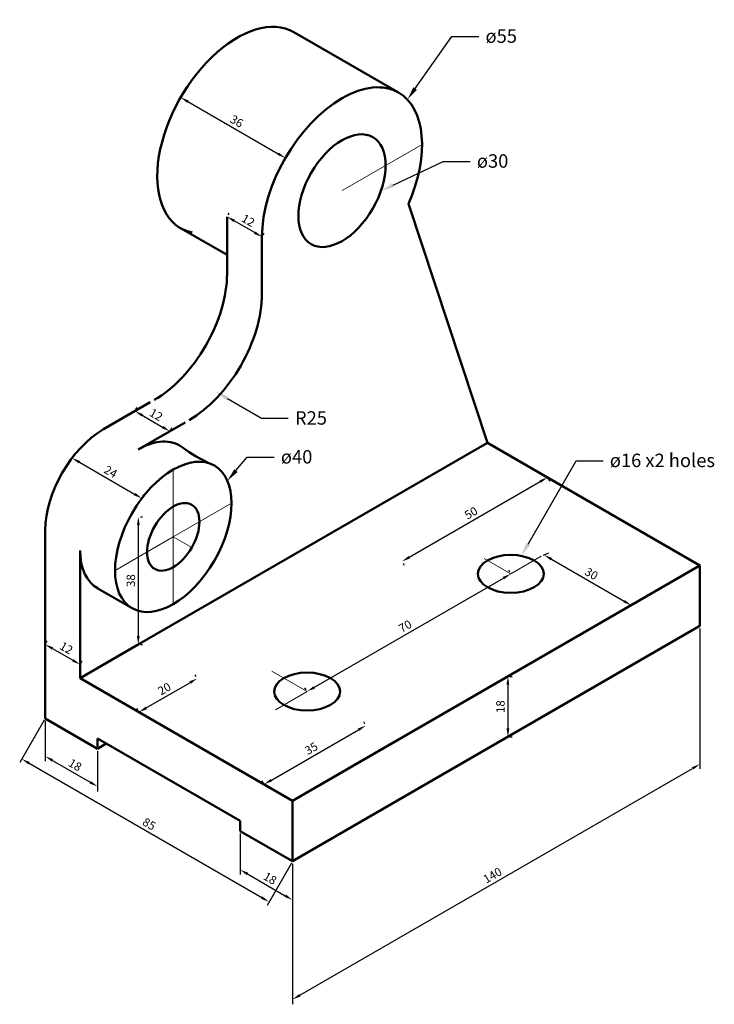
# Model space of a CAD drawing. Units: millimetres. Extents: x 2139 to 2346, y 2028 to 2321.
import ezdxf
from ezdxf import colors
from ezdxf.entities.mleader import LeaderData, LeaderLine
from ezdxf.math import Vec2, Vec3

# ---------------------------------------------------------------- set-up
doc = ezdxf.new("R2010")
doc.units = ezdxf.units.MM
doc.linetypes.add('CENTER', pattern=[50.8, 31.75, -6.35, 6.35, -6.35])
for name, color, linetype, lineweight in [('M-CNTR', 1, 'CENTER', 18), ('M-DIMS', 2, 'Continuous', 25), ('M-OUTL', 7, 'Continuous', 50), ('M-TEXT', 3, 'Continuous', 25)]:
    doc.layers.add(name, color=color, linetype=linetype, lineweight=lineweight)
doc.styles.get("Standard").update_dxf_attribs({"font": 'arial.ttf'})
doc.dimstyles.new('ISO-25', dxfattribs={"dimtxt": 2.5, "dimasz": 2.5, "dimexe": 1.25, "dimexo": 0.625, "dimtad": 1, "dimtxsty": 'Standard', "dimcen": 2.5, "dimadec": 0, "dimazin": 0, "dimtfac": 1, "dimtmove": 0, "dimatfit": 3, "dimfxl": 1, "dimarcsym": 0})

# ---------------------------------------------------------------- blocks, each defined once
blk = doc.blocks.new('*D1')
at = {"layer": 'Defpoints', "color": 0, "transparency": 16777216}
for p in [(2186.84, 2297.97), (2218.02, 2279.97), (2218.02, 2279.97)]:
    blk.add_point(p, dxfattribs=at)
at = {"layer": 'M-DIMS', "color": 0, "lineweight": -2, "transparency": 16777216}
for p, q in [((2187.16, 2298.51), (2187.47, 2299.05)), ((2189.01, 2296.72), (2215.86, 2281.22)), ((2218.33, 2280.51), (2218.65, 2281.05))]:
    blk.add_line(p, q, dxfattribs=at)
at = {"layer": 'M-DIMS', "color": 0, "transparency": 16777216}
for points in [[(2189.22, 2297.08), (2188.8, 2296.36), (2186.84, 2297.97)], [(2216.06, 2281.58), (2215.65, 2280.86), (2218.02, 2279.97)]]:
    blk.add_solid(points, dxfattribs=at)
at = {"layer": 'M-DIMS', "color": 0, "transparency": 16777216, "insert": (2203.38, 2290.62), "char_height": 2.5, "attachment_point": 5, "rotation": 330}
blk.add_mtext('36', dxfattribs=at)
blk = doc.blocks.new('*D2')
at = {"layer": 'Defpoints', "color": 0, "transparency": 16777216}
for p in [(2296.01, 2184.94), (2296.01, 2184.94), (2252.71, 2159.94)]:
    blk.add_point(p, dxfattribs=at)
at = {"layer": 'M-DIMS', "color": 0, "lineweight": -2, "transparency": 16777216}
for p, q in [((2254.87, 2161.19), (2293.84, 2183.69)), ((2296.32, 2184.4), (2296.63, 2183.86)), ((2253.02, 2159.4), (2253.33, 2158.86))]:
    blk.add_line(p, q, dxfattribs=at)
at = {"layer": 'M-DIMS', "color": 0, "transparency": 16777216}
for points in [[(2293.64, 2184.05), (2294.05, 2183.33), (2296.01, 2184.94)], [(2254.66, 2161.55), (2255.08, 2160.83), (2252.71, 2159.94)]]:
    blk.add_solid(points, dxfattribs=at)
at = {"layer": 'M-DIMS', "color": 0, "transparency": 16777216, "insert": (2273.41, 2174.09), "char_height": 2.5, "attachment_point": 5, "rotation": 30}
blk.add_mtext('50', dxfattribs=at)
blk = doc.blocks.new('*D3')
at = {"layer": 'Defpoints', "color": 0, "transparency": 16777216}
for p in [(2241.97, 2111.14), (2241.97, 2111.14), (2211.66, 2093.64)]:
    blk.add_point(p, dxfattribs=at)
at = {"layer": 'M-DIMS', "color": 0, "lineweight": -2, "transparency": 16777216}
for p, q in [((2241.66, 2111.68), (2241.35, 2112.22)), ((2213.83, 2094.89), (2239.81, 2109.89)), ((2211.35, 2094.18), (2211.04, 2094.72))]:
    blk.add_line(p, q, dxfattribs=at)
at = {"layer": 'M-DIMS', "color": 0, "transparency": 16777216}
for points in [[(2239.6, 2110.25), (2240.01, 2109.53), (2241.97, 2111.14)], [(2213.62, 2095.25), (2214.03, 2094.53), (2211.66, 2093.64)]]:
    blk.add_solid(points, dxfattribs=at)
at = {"layer": 'M-DIMS', "color": 0, "transparency": 16777216, "insert": (2225.86, 2104.04), "char_height": 2.5, "attachment_point": 5, "rotation": 30}
blk.add_mtext('35', dxfattribs=at)
blk = doc.blocks.new('*D4')
at = {"layer": 'Defpoints', "color": 0, "transparency": 16777216}
for p in [(2146.53, 2113.25), (2162.12, 2104.25), (2162.12, 2092.99)]:
    blk.add_point(p, dxfattribs=at)
at = {"layer": 'M-DIMS', "color": 0, "lineweight": -2, "transparency": 16777216}
for p, q in [((2146.53, 2112.52), (2146.53, 2100.54)), ((2162.12, 2103.52), (2162.12, 2091.54)), ((2148.69, 2100.74), (2159.95, 2094.24))]:
    blk.add_line(p, q, dxfattribs=at)
at = {"layer": 'M-DIMS', "color": 0, "transparency": 16777216}
for points in [[(2148.9, 2101.1), (2148.48, 2100.37), (2146.53, 2101.99)], [(2160.16, 2094.6), (2159.74, 2093.87), (2162.12, 2092.99)]]:
    blk.add_solid(points, dxfattribs=at)
at = {"layer": 'M-DIMS', "color": 0, "transparency": 16777216, "insert": (2155.27, 2099.13), "char_height": 2.5, "attachment_point": 5, "rotation": 330}
blk.add_mtext('18', dxfattribs=at)
blk = doc.blocks.new('*D5')
at = {"layer": 'Defpoints', "color": 0, "transparency": 16777216}
for p in [(2204.55, 2079.75), (2220.14, 2070.75), (2220.14, 2059.24)]:
    blk.add_point(p, dxfattribs=at)
at = {"layer": 'M-DIMS', "color": 0, "lineweight": -2, "transparency": 16777216}
for p, q in [((2204.55, 2079.02), (2204.55, 2066.8)), ((2220.14, 2070.02), (2220.14, 2057.8)), ((2206.72, 2066.99), (2217.97, 2060.49))]:
    blk.add_line(p, q, dxfattribs=at)
at = {"layer": 'M-DIMS', "color": 0, "transparency": 16777216}
for points in [[(2206.92, 2067.35), (2206.51, 2066.63), (2204.55, 2068.24)], [(2218.18, 2060.85), (2217.77, 2060.13), (2220.14, 2059.24)]]:
    blk.add_solid(points, dxfattribs=at)
at = {"layer": 'M-DIMS', "color": 0, "transparency": 16777216, "insert": (2213.3, 2065.39), "char_height": 2.5, "attachment_point": 5, "rotation": 330}
blk.add_mtext('18', dxfattribs=at)
blk = doc.blocks.new('*D6')
at = {"layer": 'Defpoints', "color": 0, "transparency": 16777216}
for p in [(2341.38, 2140.75), (2341.38, 2099.64), (2220.14, 2070.75)]:
    blk.add_point(p, dxfattribs=at)
at = {"layer": 'M-DIMS', "color": 0, "lineweight": -2, "transparency": 16777216}
for p, q in [((2341.38, 2140.02), (2341.38, 2098.2)), ((2222.3, 2030.89), (2339.22, 2098.39)), ((2220.14, 2070.02), (2220.14, 2028.2))]:
    blk.add_line(p, q, dxfattribs=at)
at = {"layer": 'M-DIMS', "color": 0, "transparency": 16777216}
for points in [[(2339.01, 2098.75), (2339.43, 2098.03), (2341.38, 2099.64)], [(2222.1, 2031.25), (2222.51, 2030.53), (2220.14, 2029.64)]]:
    blk.add_solid(points, dxfattribs=at)
at = {"layer": 'M-DIMS', "color": 0, "transparency": 16777216, "insert": (2279.81, 2066.29), "char_height": 2.5, "attachment_point": 5, "rotation": 30}
blk.add_mtext('140', dxfattribs=at)
blk = doc.blocks.new('*D7')
at = {"layer": 'Defpoints', "color": 0, "transparency": 16777216}
for p in [(2294.14, 2161.47), (2320.12, 2146.47), (2320.98, 2146.87)]:
    blk.add_point(p, dxfattribs=at)
at = {"layer": 'M-DIMS', "color": 0, "lineweight": -2, "transparency": 16777216}
for p, q in [((2294.83, 2161.79), (2296.39, 2162.52)), ((2297.17, 2160.62), (2318.82, 2148.12)), ((2320.81, 2146.79), (2322.37, 2147.52))]:
    blk.add_line(p, q, dxfattribs=at)
at = {"layer": 'M-DIMS', "color": 0, "transparency": 16777216}
for points in [[(2297.38, 2160.98), (2296.96, 2160.26), (2295, 2161.87)], [(2319.03, 2148.48), (2318.61, 2147.76), (2320.98, 2146.87)]]:
    blk.add_solid(points, dxfattribs=at)
at = {"layer": 'M-DIMS', "color": 0, "transparency": 16777216, "insert": (2308.94, 2156.02), "char_height": 2.5, "attachment_point": 5, "rotation": 330}
blk.add_mtext('30', dxfattribs=at)
blk = doc.blocks.new('*D8')
at = {"layer": 'Defpoints', "color": 0, "transparency": 16777216}
for p in [(2173.24, 2204.67), (2183.63, 2198.67), (2183.63, 2198.67)]:
    blk.add_point(p, dxfattribs=at)
at = {"layer": 'M-DIMS', "color": 0, "lineweight": -2, "transparency": 16777216}
for p, q in [((2173.55, 2205.21), (2173.87, 2205.75)), ((2175.41, 2203.42), (2181.47, 2199.92)), ((2183.95, 2199.21), (2184.26, 2199.75))]:
    blk.add_line(p, q, dxfattribs=at)
at = {"layer": 'M-DIMS', "color": 0, "transparency": 16777216}
for points in [[(2175.62, 2203.78), (2175.2, 2203.06), (2173.24, 2204.67)], [(2181.68, 2200.28), (2181.26, 2199.56), (2183.63, 2198.67)]]:
    blk.add_solid(points, dxfattribs=at)
at = {"layer": 'M-DIMS', "color": 0, "transparency": 16777216, "insert": (2179.38, 2203.3), "char_height": 2.5, "attachment_point": 5, "rotation": 330}
blk.add_mtext('12', dxfattribs=at)
blk = doc.blocks.new('*D9')
at = {"layer": 'Defpoints', "color": 0, "transparency": 16777216}
for p in [(2154.52, 2190.72), (2175.31, 2178.72), (2175.31, 2178.72)]:
    blk.add_point(p, dxfattribs=at)
at = {"layer": 'M-DIMS', "color": 0, "lineweight": -2, "transparency": 16777216}
for p, q in [((2154.83, 2191.26), (2155.15, 2191.8)), ((2156.69, 2189.47), (2173.14, 2179.97)), ((2175.62, 2179.26), (2175.93, 2179.8))]:
    blk.add_line(p, q, dxfattribs=at)
at = {"layer": 'M-DIMS', "color": 0, "transparency": 16777216}
for points in [[(2156.9, 2189.83), (2156.48, 2189.1), (2154.52, 2190.72)], [(2173.35, 2180.33), (2172.93, 2179.6), (2175.31, 2178.72)]]:
    blk.add_solid(points, dxfattribs=at)
at = {"layer": 'M-DIMS', "color": 0, "transparency": 16777216, "insert": (2165.85, 2186.34), "char_height": 2.5, "attachment_point": 5, "rotation": 330}
blk.add_mtext('24', dxfattribs=at)
blk = doc.blocks.new('*D10')
at = {"layer": 'Defpoints', "color": 0, "transparency": 16777216}
for p in [(2146.53, 2135.28), (2156.92, 2129.28), (2156.92, 2129.28)]:
    blk.add_point(p, dxfattribs=at)
at = {"layer": 'M-DIMS', "color": 0, "lineweight": -2, "transparency": 16777216}
for p, q in [((2146.84, 2135.82), (2147.15, 2136.36)), ((2148.69, 2134.03), (2154.75, 2130.53)), ((2157.23, 2129.82), (2157.54, 2130.36))]:
    blk.add_line(p, q, dxfattribs=at)
at = {"layer": 'M-DIMS', "color": 0, "transparency": 16777216}
for points in [[(2148.9, 2134.39), (2148.48, 2133.67), (2146.53, 2135.28)], [(2154.96, 2130.89), (2154.55, 2130.17), (2156.92, 2129.28)]]:
    blk.add_solid(points, dxfattribs=at)
at = {"layer": 'M-DIMS', "color": 0, "transparency": 16777216, "insert": (2152.66, 2133.91), "char_height": 2.5, "attachment_point": 5, "rotation": 330}
blk.add_mtext('12', dxfattribs=at)
blk = doc.blocks.new('*D11')
at = {"layer": 'Defpoints', "color": 0, "transparency": 16777216}
for p in [(2284.24, 2125.75), (2284.24, 2107.75), (2284.24, 2107.75)]:
    blk.add_point(p, dxfattribs=at)
at = {"layer": 'M-DIMS', "color": 0, "lineweight": -2, "transparency": 16777216}
for p, q in [((2284.86, 2125.75), (2285.49, 2125.75)), ((2284.24, 2123.25), (2284.24, 2110.25)), ((2284.86, 2107.75), (2285.49, 2107.75))]:
    blk.add_line(p, q, dxfattribs=at)
at = {"layer": 'M-DIMS', "color": 0, "transparency": 16777216}
for points in [[(2283.82, 2123.25), (2284.66, 2123.25), (2284.24, 2125.75)], [(2283.82, 2110.25), (2284.66, 2110.25), (2284.24, 2107.75)]]:
    blk.add_solid(points, dxfattribs=at)
at = {"layer": 'M-DIMS', "color": 0, "transparency": 16777216, "insert": (2282.34, 2116.75), "char_height": 2.5, "attachment_point": 5, "rotation": 90}
blk.add_mtext('18', dxfattribs=at)
blk = doc.blocks.new('*D12')
at = {"layer": 'Defpoints', "color": 0, "transparency": 16777216}
for p in [(2191.77, 2125.13), (2191.77, 2125.13), (2174.45, 2115.13)]:
    blk.add_point(p, dxfattribs=at)
at = {"layer": 'M-DIMS', "color": 0, "lineweight": -2, "transparency": 16777216}
for p, q in [((2176.61, 2116.38), (2189.6, 2123.88)), ((2191.46, 2125.67), (2191.14, 2126.21)), ((2174.14, 2115.67), (2173.82, 2116.21))]:
    blk.add_line(p, q, dxfattribs=at)
at = {"layer": 'M-DIMS', "color": 0, "transparency": 16777216}
for points in [[(2189.4, 2124.24), (2189.81, 2123.51), (2191.77, 2125.13)], [(2176.41, 2116.74), (2176.82, 2116.01), (2174.45, 2115.13)]]:
    blk.add_solid(points, dxfattribs=at)
at = {"layer": 'M-DIMS', "color": 0, "transparency": 16777216, "insert": (2182.16, 2121.77), "char_height": 2.5, "attachment_point": 5, "rotation": 30}
blk.add_mtext('20', dxfattribs=at)
blk = doc.blocks.new('*D13')
at = {"layer": 'Defpoints', "color": 0, "transparency": 16777216}
for p in [(2200.65, 2262.5), (2211.05, 2256.5), (2211.05, 2256.5)]:
    blk.add_point(p, dxfattribs=at)
at = {"layer": 'M-DIMS', "color": 0, "lineweight": -2, "transparency": 16777216}
for p, q in [((2200.97, 2263.04), (2201.28, 2263.58)), ((2202.82, 2261.25), (2208.88, 2257.75)), ((2211.36, 2257.04), (2211.67, 2257.58))]:
    blk.add_line(p, q, dxfattribs=at)
at = {"layer": 'M-DIMS', "color": 0, "transparency": 16777216}
for points in [[(2203.03, 2261.61), (2202.61, 2260.88), (2200.65, 2262.5)], [(2209.09, 2258.11), (2208.67, 2257.38), (2211.05, 2256.5)]]:
    blk.add_solid(points, dxfattribs=at)
at = {"layer": 'M-DIMS', "color": 0, "transparency": 16777216, "insert": (2206.79, 2261.12), "char_height": 2.5, "attachment_point": 5, "rotation": 330}
blk.add_mtext('12', dxfattribs=at)
blk = doc.blocks.new('*D14')
at = {"layer": 'Defpoints', "color": 0, "transparency": 16777216}
for p in [(2285.09, 2156.25), (2285.09, 2156.25), (2224.47, 2121.25)]:
    blk.add_point(p, dxfattribs=at)
at = {"layer": 'M-DIMS', "color": 0, "lineweight": -2, "transparency": 16777216}
for p, q in [((2284.78, 2156.79), (2284.47, 2157.33)), ((2226.63, 2122.5), (2282.93, 2155)), ((2224.16, 2121.79), (2223.84, 2122.33))]:
    blk.add_line(p, q, dxfattribs=at)
at = {"layer": 'M-DIMS', "color": 0, "transparency": 16777216}
for points in [[(2282.72, 2155.36), (2283.13, 2154.63), (2285.09, 2156.25)], [(2226.43, 2122.86), (2226.84, 2122.13), (2224.47, 2121.25)]]:
    blk.add_solid(points, dxfattribs=at)
at = {"layer": 'M-DIMS', "color": 0, "transparency": 16777216, "insert": (2253.83, 2140.39), "char_height": 2.5, "attachment_point": 5, "rotation": 30}
blk.add_mtext('70', dxfattribs=at)
blk = doc.blocks.new('*D15')
at = {"layer": 'Defpoints', "color": 0, "transparency": 16777216}
for p in [(2146.53, 2113.25), (2220.14, 2070.75), (2213.17, 2058.68)]:
    blk.add_point(p, dxfattribs=at)
at = {"layer": 'M-DIMS', "color": 0, "lineweight": -2, "transparency": 16777216}
for p, q in [((2146.21, 2112.7), (2138.93, 2100.09)), ((2141.72, 2099.93), (2211.01, 2059.93)), ((2219.83, 2070.2), (2212.55, 2057.59))]:
    blk.add_line(p, q, dxfattribs=at)
at = {"layer": 'M-DIMS', "color": 0, "transparency": 16777216}
for points in [[(2141.93, 2100.29), (2141.52, 2099.57), (2139.56, 2101.18)], [(2211.21, 2060.29), (2210.8, 2059.57), (2213.17, 2058.68)]]:
    blk.add_solid(points, dxfattribs=at)
at = {"layer": 'M-DIMS', "color": 0, "transparency": 16777216, "insert": (2177.32, 2081.57), "char_height": 2.5, "attachment_point": 5, "rotation": 330}
blk.add_mtext('85', dxfattribs=at)
blk = doc.blocks.new('*D16')
at = {"layer": 'Defpoints', "color": 0, "transparency": 16777216}
for p in [(2174.24, 2173.25), (2174.24, 2135.25), (2174.24, 2135.25)]:
    blk.add_point(p, dxfattribs=at)
at = {"layer": 'M-DIMS', "color": 0, "lineweight": -2, "transparency": 16777216}
for p, q in [((2174.24, 2170.75), (2174.24, 2137.75)), ((2174.86, 2173.25), (2175.49, 2173.25)), ((2174.86, 2135.25), (2175.49, 2135.25))]:
    blk.add_line(p, q, dxfattribs=at)
at = {"layer": 'M-DIMS', "color": 0, "transparency": 16777216}
for points in [[(2173.82, 2170.75), (2174.66, 2170.75), (2174.24, 2173.25)], [(2173.82, 2137.75), (2174.66, 2137.75), (2174.24, 2135.25)]]:
    blk.add_solid(points, dxfattribs=at)
at = {"layer": 'M-DIMS', "color": 0, "transparency": 16777216, "insert": (2172.34, 2154.25), "char_height": 2.5, "attachment_point": 5, "rotation": 90}
blk.add_mtext('38', dxfattribs=at)

msp = doc.modelspace()

# ---------------------------------------------------------------- linework, layer by layer
at = {"layer": 'M-CNTR'}
for p, q in [((2234.862, 2270.246), (2258.677, 2283.996)), ((2184.632, 2167.246), (2184.632, 2187.246)), ((2184.632, 2167.246), (2201.953, 2177.246)), ((2184.632, 2167.246), (2167.312, 2157.246)), ((2184.632, 2167.246), (2184.632, 2147.246)), ((2184.632, 2167.246), (2190.143, 2164.064)), ((2285.091, 2156.246), (2277.151, 2160.83)), ((2285.091, 2156.246), (2294.138, 2161.469)), ((2285.091, 2156.246), (2275.819, 2150.892)), ((2224.469, 2121.246), (2213.963, 2127.312)), ((2231.398, 2125.246), (2232.942, 2126.137)), ((2224.469, 2121.246), (2215.083, 2115.827))]:
    msp.add_line(p, q, dxfattribs=at)
at = {"layer": 'M-OUTL'}
for p, q in [((2251.703, 2299.414), (2220.525, 2317.414)), ((2278.163, 2195.246), (2254.615, 2266.289)), ((2200.654, 2262.496), (2200.654, 2245.496)), ((2200.654, 2251.105), (2186.845, 2259.078)), ((2211.046, 2256.496), (2211.046, 2239.496)), ((2163.848, 2199.246), (2177.761, 2207.279)), ((2174.24, 2193.246), (2188.154, 2201.279)), ((2174.24, 2135.246), (2278.163, 2195.246)), ((2278.163, 2195.246), (2341.383, 2158.746)), ((2146.527, 2169.246), (2146.527, 2131.246)), ((2146.527, 2131.246), (2146.527, 2169.246)), ((2156.919, 2125.246), (2156.919, 2163.246)), ((2220.139, 2088.746), (2341.383, 2158.746)), ((2341.383, 2158.746), (2341.383, 2140.746)), ((2172.385, 2146.033), (2161.992, 2152.033)), ((2341.383, 2140.746), (2220.139, 2070.746)), ((2156.919, 2125.246), (2174.24, 2135.246)), ((2146.527, 2113.246), (2146.527, 2131.246)), ((2156.919, 2125.246), (2220.139, 2088.746)), ((2156.919, 2125.246), (2167.312, 2119.246)), ((2146.527, 2113.246), (2162.115, 2104.246)), ((2162.115, 2104.246), (2162.115, 2107.246)), ((2204.551, 2082.746), (2162.115, 2107.246)), ((2220.139, 2088.746), (2250.45, 2106.246)), ((2162.116, 2104.246), (2164.714, 2105.746)), ((2220.139, 2070.746), (2220.139, 2088.746)), ((2204.551, 2079.746), (2204.551, 2082.746)), ((2220.139, 2070.746), (2204.551, 2079.746)), ((2220.139, 2070.746), (2204.551, 2079.746)), ((2204.551, 2079.746), (2220.139, 2070.746))]:
    msp.add_line(p, q, dxfattribs=at)
msp.add_arc((2211.496, 2225.775), 40, 232.85031, 247.14969, dxfattribs=at)
for centre, major_axis, start_param, end_param in [((2203.685, 2288.246), (-16.84, -29.168), 3.1415983, 6.469802), ((2234.862, 2270.246), (16.84, 29.168), 0, 0.7853982), ((2234.862, 2270.246), (16.84, 29.168), 4.9050601, 6.2831853), ((2234.862, 2270.246), (16.84, 29.168), 0.7853982, 2.3561945), ((2179.004, 2232.995), (15.309, 26.515), 3.9269457, 5.4978323), ((2189.396, 2226.995), (15.309, 26.515), 3.9269457, 5.4978323), ((2163.848, 2179.246), (-12.247, -21.213), 3.9269908, 5.4977871), ((2174.24, 2173.246), (-12.247, -21.213), 9.3524828, 10.2101761), ((2174.24, 2173.246), (-12.247, -21.213), 5.4977871, 6.304756)]:
    msp.add_ellipse(centre, major_axis=major_axis, ratio=0.5773503, start_param=start_param, end_param=end_param, dxfattribs=at)
for centre, major_axis in [((2234.862, 2270.246), (-9.186, -15.91)), ((2184.632, 2167.246), (-12.247, -21.213)), ((2184.632, 2167.246), (-12.247, -21.213)), ((2184.632, 2167.246), (-5.511, -9.546)), ((2285.091, 2156.246), (-9.798, 0)), ((2224.469, 2121.246), (-9.798, 0))]:
    msp.add_ellipse(centre, major_axis=major_axis, ratio=0.5773503, dxfattribs=at)

# ---------------------------------------------------------------- dimensions: what is measured, and where the dimension line sits
at = {"layer": 'M-DIMS'}
for p1, p2, distance, picture, middle in [((2186.844, 2297.969), (2218.021, 2279.969), 0, '*D1', (2203.384, 2290.616)), ((2200.654, 2262.496), (2211.046, 2256.496), 0, '*D13', (2206.79, 2261.124)), ((2173.242, 2204.67), (2183.634, 2198.67), 0, '*D8', (2179.378, 2203.298)), ((2154.522, 2190.715), (2175.307, 2178.715), 0, '*D9', (2165.854, 2186.344)), ((2252.708, 2159.942), (2296.009, 2184.942), 0, '*D2', (2273.408, 2174.089)), ((2294.138, 2161.469), (2320.118, 2146.469), 0.782, '*D7', (2308.944, 2156.019)), ((2220.139, 2070.746), (2341.383, 2140.746), -35.597, '*D6', (2279.81, 2066.289)), ((2146.527, 2135.281), (2156.919, 2129.281), 0, '*D10', (2152.663, 2133.91)), ((2174.449, 2115.125), (2191.769, 2125.125), 0, '*D12', (2182.158, 2121.772)), ((2284.24, 2125.754), (2284.24, 2107.754), 0, '*D11', (2282.339, 2116.754)), ((2146.527, 2113.246), (2162.115, 2104.246), -9.752, '*D4', (2155.272, 2099.132)), ((2211.66, 2093.641), (2241.971, 2111.141), 0, '*D3', (2225.864, 2104.039)), ((2204.551, 2079.746), (2220.139, 2070.746), -9.961, '*D5', (2213.296, 2065.391))]:
    dim = msp.add_aligned_dim(p1=p1, p2=p2, distance=distance, dimstyle='ISO-25', override={"dimclrd": 0, "dimclre": 0, "dimclrt": 0}, dxfattribs=at)
    dim.commit()
    dim.dimension.update_dxf_attribs({"geometry": picture, "text_midpoint": middle})
for base, p1, p2, angle, picture, middle in [((2174.24, 2135.246), (2174.24, 2173.246), (2174.24, 2135.246), 270, '*D16', (2172.338, 2154.246)), ((2285.091, 2156.246), (2224.469, 2121.246), (2285.091, 2156.246), 30, '*D14', (2253.829, 2140.392)), ((2213.171, 2058.677), (2146.527, 2113.246), (2220.139, 2070.746), 330, '*D15', (2177.316, 2081.574))]:
    dim = msp.add_linear_dim(base=base, p1=p1, p2=p2, angle=angle, dimstyle='ISO-25', override={"dimrnd": 0}, dxfattribs=at)
    dim.commit()
    dim.dimension.update_dxf_attribs({"geometry": picture, "text_midpoint": middle})

# ---------------------------------------------------------------- leaders
at = {"layer": 'M-TEXT'}
ml = msp.add_multileader_mtext('Standard', dxfattribs=at)
ml.set_content('ø55', color=256)
ml.set_leader_properties()
ml.build(insert=Vec2(0, 0))
ctx = ml.context
ctx.base_point, ctx.plane_origin = Vec3(2275.575, 2316.121), Vec3(2254.323, 2297.332)
notes = []
notes.append((ctx, [(0, (1, 1, 0), (2267.575, 2316.121), (1, 0), 8, [(0, [(2254.323, 2297.332)], 0, [])])]))
ctx.mtext.insert, ctx.mtext.flow_direction = Vec3(2277.575, 2318.228), 5
ml = msp.add_multileader_mtext('Standard', dxfattribs=at)
ml.set_content('ø30', color=256)
ml.set_leader_properties()
ml.build(insert=Vec2(0, 0))
ctx = ml.context
ctx.base_point, ctx.plane_origin = Vec3(2273.008, 2278.964), Vec3(2246.439, 2270.128)
notes.append((ctx, [(0, (1, 1, 0), (2265.008, 2278.964), (1, 0), 8, [(0, [(2246.439, 2270.128)], 0, [])])]))
ctx.mtext.insert, ctx.mtext.flow_direction = Vec3(2275.008, 2281.072), 5
ml = msp.add_multileader_mtext('Standard', dxfattribs=at)
ml.set_content('R25', color=256)
ml.set_leader_properties()
ml.build(insert=Vec2(0, 0))
ctx = ml.context
ctx.base_point, ctx.plane_origin = Vec3(2218.868, 2202.598), Vec3(2197.304, 2210.43)
notes.append((ctx, [(0, (1, 1, 0), (2210.868, 2202.598), (1, 0), 8, [(0, [(2197.304, 2210.43)], 0, [])])]))
ctx.mtext.insert, ctx.mtext.flow_direction = Vec3(2220.868, 2204.632), 5
ml = msp.add_multileader_mtext('Standard', dxfattribs=at)
ml.set_content('ø40', color=256)
ml.set_leader_properties()
ml.build(insert=Vec2(0, 0))
ctx = ml.context
ctx.base_point, ctx.plane_origin = Vec3(2214.678, 2190.962), Vec3(2200.731, 2183.918)
notes.append((ctx, [(0, (1, 1, 0), (2206.678, 2190.962), (1, 0), 8, [(0, [(2200.731, 2183.918)], 0, [])])]))
ctx.mtext.insert, ctx.mtext.flow_direction = Vec3(2216.678, 2193.07), 5
ml = msp.add_multileader_mtext('Standard', dxfattribs=at)
ml.set_content('ø16 x2 holes', color=256)
ml.set_leader_properties()
ml.build(insert=Vec2(0, 0))
ctx = ml.context
ctx.base_point, ctx.plane_origin = Vec3(2312.57, 2189.901), Vec3(2288.233, 2161.604)
notes.append((ctx, [(0, (1, 1, 0), (2304.57, 2189.901), (1, 0), 8, [(0, [(2288.233, 2161.604)], 0, [])])]))
ctx.mtext.insert, ctx.mtext.flow_direction = Vec3(2314.57, 2192.009), 5
for ctx, leaders in notes:
    for number, flags, end, landing, length, lines in leaders:
        leader = LeaderData()
        leader.index, (leader.has_last_leader_line, leader.has_dogleg_vector, leader.attachment_direction) = number, flags
        leader.last_leader_point, leader.dogleg_vector, leader.dogleg_length = Vec3(end), Vec3(landing), length
        for number, points, colour, breaks in lines:
            line = LeaderLine()
            line.index, line.vertices, line.color, line.breaks = number, Vec3.list(points), colors.encode_raw_color(colour), breaks
            leader.lines.append(line)
        ctx.leaders.append(leader)

doc.saveas('drawing.dxf')
